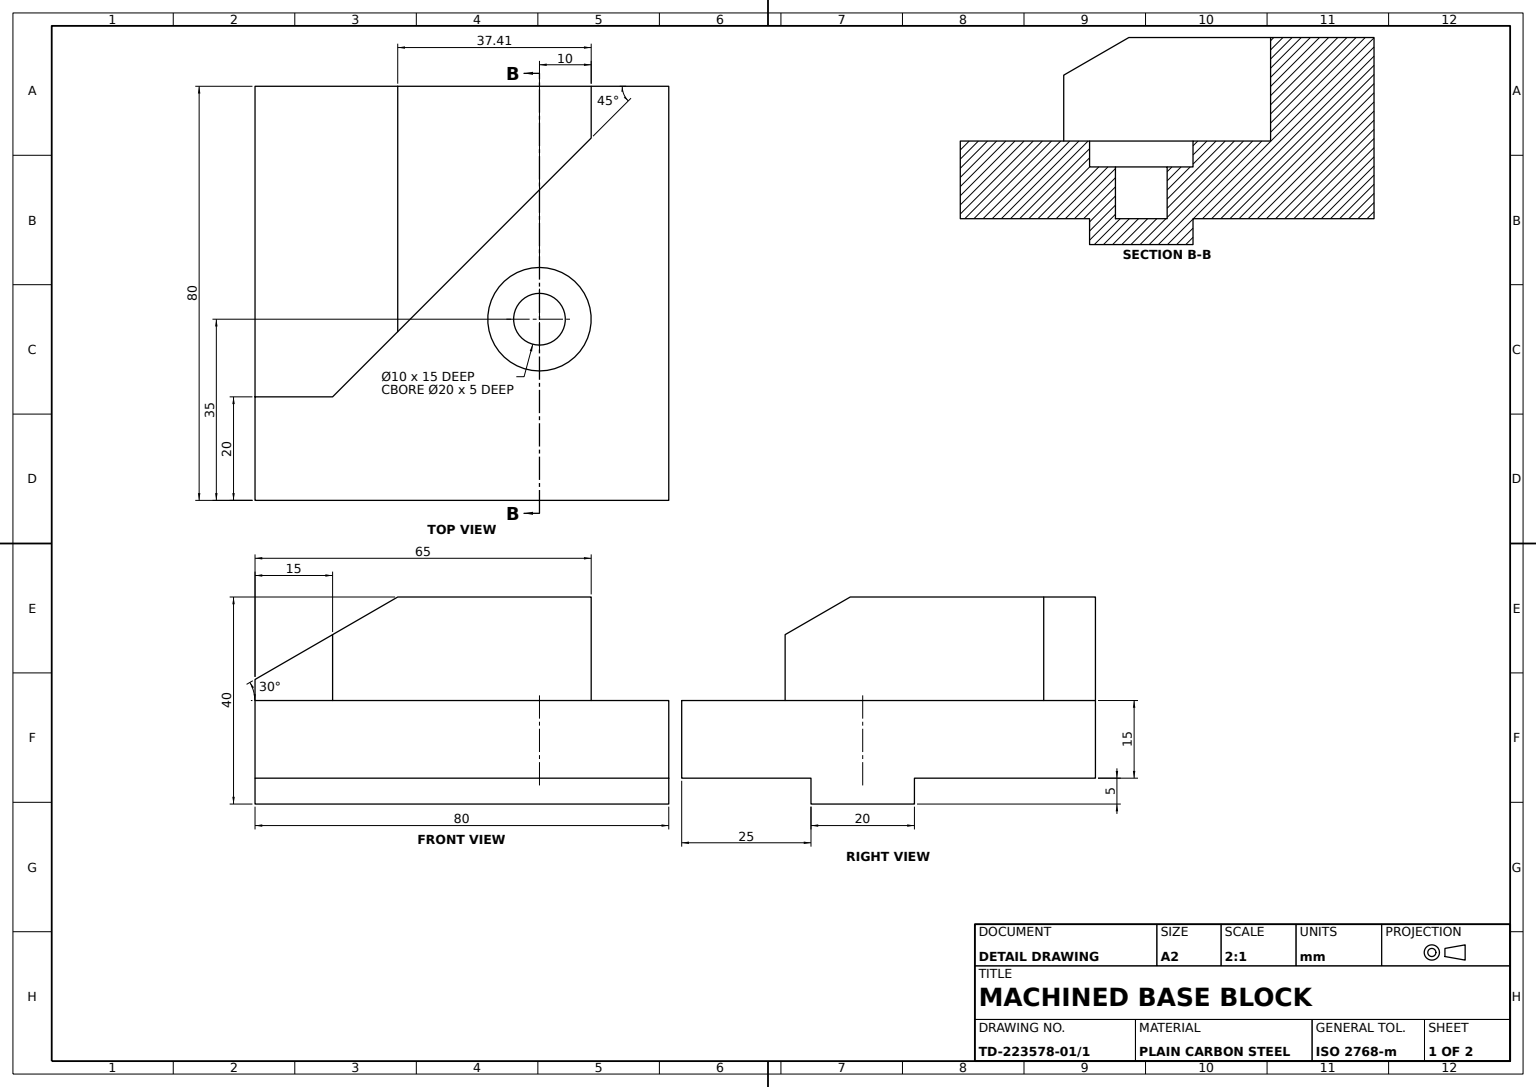
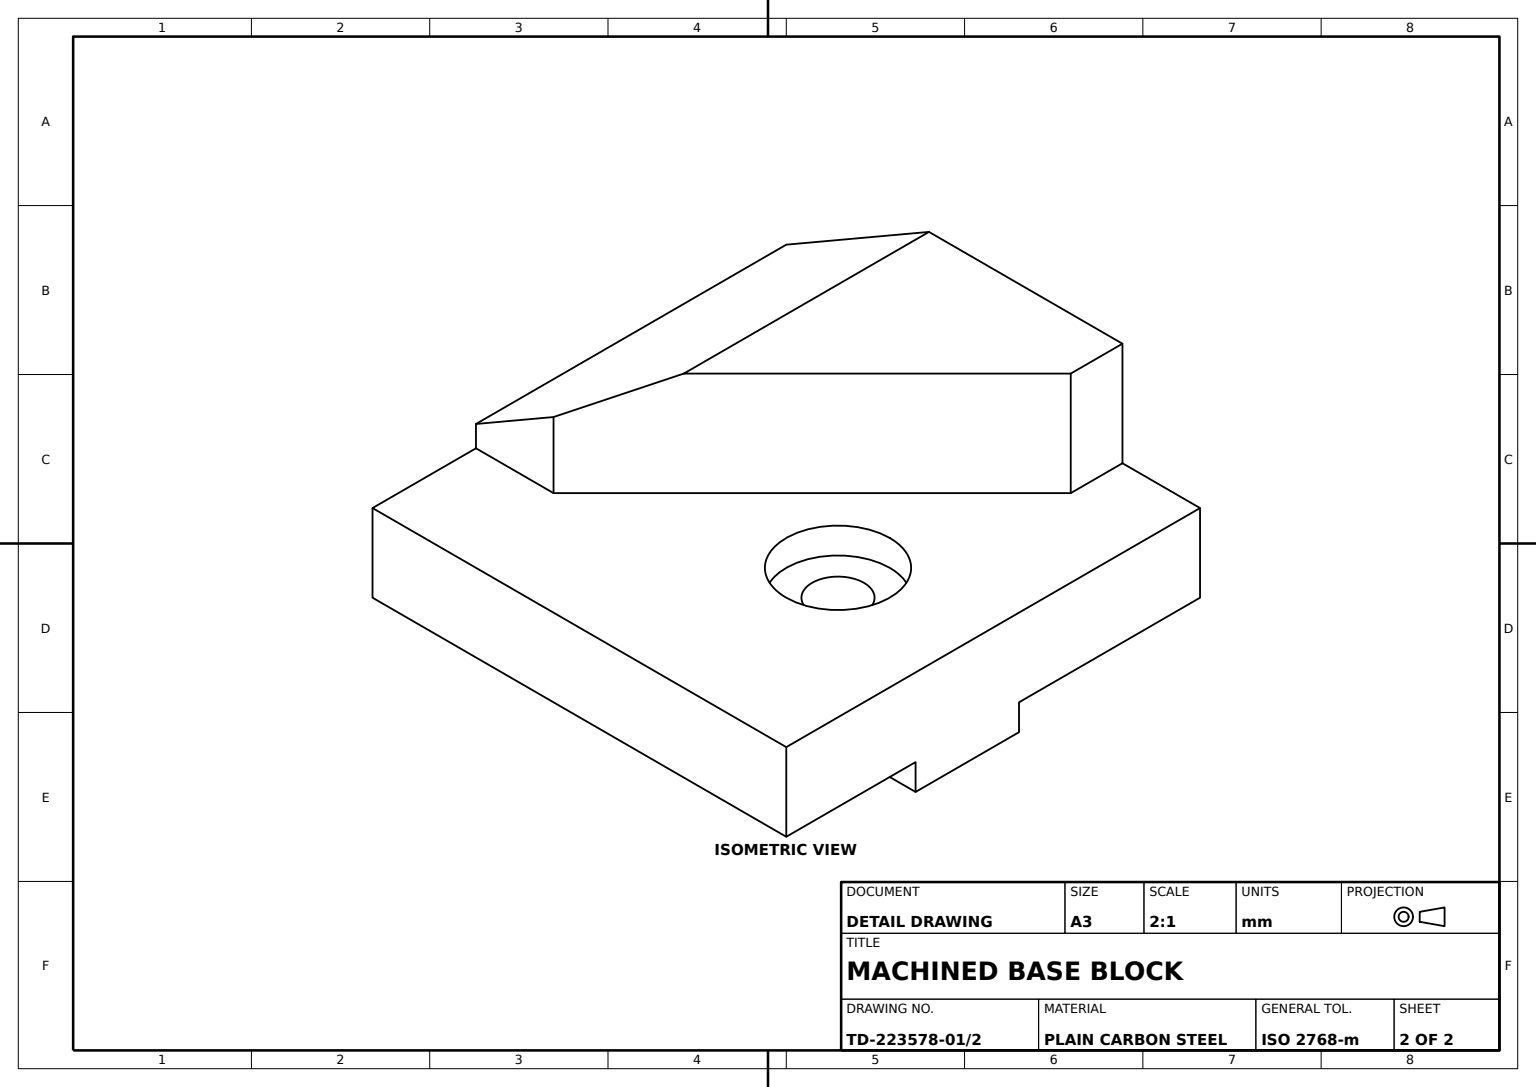
from build123d import *

# Parameters (mm, degrees)
BASE_PLATE_SKETCH_W          = 80
BASE_PLATE_SKETCH_H          = 80
BASE_PLATE_80X80X20_DEPTH    = 20
BOTTOM_SLOT_SKETCH_W         = 25
BOTTOM_SLOT_SKETCH_H         = 5
BOTTOM_SLOT_SKETCH_W_2       = 35
BOTTOM_SLOT_DEPTH            = 80
RAISED_BLOCK_SKETCH_W        = 80
RAISED_BLOCK_SKETCH_H        = 60
RAISED_BLOCK_DEPTH           = 20
BLOCK_STEP_CUT_1_SKETCH_W    = 15
BLOCK_STEP_CUT_1_SKETCH_H    = 10
BLOCK_STEP_CUT_1_DEPTH       = 20
BLOCK_STEP_CUT_2_DEPTH       = 20
BLOCK_ANGLE_CUT_30DEG_REACH  = 102.233
COUNTERBORE_25_SKETCH_R      = 10
COUNTERBORE_25X5_DEPTH       = 5
HOLE_10_SKETCH_R             = 5
HOLE_10X10_DEPTH             = 10
AUXILIARY_BODY_EXTRUDE_DEPTH = 50
AUXILIARY_BODY_FILLET_R20_R  = 20


with BuildPart() as part:
    # Base Plate Sketch → Base Plate 80x80x20 (new body)
    with BuildSketch(Plane(origin=(0, 0, 0), x_dir=(1, 0, 0), z_dir=(0, 1, 0))):
        with Locations((5.239833721, 5.239833721)):
            Rectangle(BASE_PLATE_SKETCH_W, BASE_PLATE_SKETCH_H)
    extrude(amount=BASE_PLATE_80X80X20_DEPTH)

    # Bottom Slot Sketch → Bottom Slot (cut)
    with BuildSketch(Plane(origin=(45.239833721, 0, 0), x_dir=(0, 0, -1), z_dir=(1, 0, 0))):
        with Locations((-22.260166279, 2.5)):
            Rectangle(BOTTOM_SLOT_SKETCH_W, BOTTOM_SLOT_SKETCH_H)
        with Locations((27.739833721, 2.5)):
            Rectangle(BOTTOM_SLOT_SKETCH_W_2, BOTTOM_SLOT_SKETCH_H)
    extrude(amount=-BOTTOM_SLOT_DEPTH, mode=Mode.SUBTRACT)

    # Raised Block Sketch → Raised Block (add)
    with BuildSketch(Plane(origin=(0, 20, 0), x_dir=(1, 0, 0), z_dir=(0, 1, 0))):
        with Locations((5.239833721, 15.239833721)):
            Rectangle(RAISED_BLOCK_SKETCH_W, RAISED_BLOCK_SKETCH_H)
    extrude(amount=RAISED_BLOCK_DEPTH)

    # Block Step Cut 1 Sketch → Block Step Cut 1 (cut)
    with BuildSketch(Plane(origin=(0, 40, 0), x_dir=(1, 0, 0), z_dir=(0, 1, 0))):
        with Locations((37.739833721, 40.239833721)):
            Rectangle(BLOCK_STEP_CUT_1_SKETCH_W, BLOCK_STEP_CUT_1_SKETCH_H)
    extrude(amount=-BLOCK_STEP_CUT_1_DEPTH, mode=Mode.SUBTRACT)

    # Block Step Cut 2 Sketch → Block Step Cut 2 (cut)
    with BuildSketch(Plane(origin=(0, 40, 0), x_dir=(1, 0, 0), z_dir=(0, 1, 0))):
        Polygon((30.239833721, 35.239833721), (-19.760166279, -14.760166279), (45.239833721, -14.760166279), (45.239833721, 35.239833721), align=None)
    extrude(amount=-BLOCK_STEP_CUT_2_DEPTH, mode=Mode.SUBTRACT)

    # Block Angle Cut 30deg Sketch → Block Angle Cut 30deg (cut, up to next)
    with BuildSketch(Plane(origin=(0, 0, -45.239833721), x_dir=(-1, 0, 0), z_dir=(0, 0, -1)), mode=Mode.PRIVATE) as block_angle_cut_30deg_sk1:
        Polygon((34.760166279, 40), (7.167951709, 40), (34.760166279, 24.06962749), align=None)
    block_angle_cut_30deg_tool1 = extrude(block_angle_cut_30deg_sk1.sketch, amount=-BLOCK_ANGLE_CUT_30DEG_REACH, mode=Mode.PRIVATE) & part.part
    add(block_angle_cut_30deg_tool1.solids().sort_by_distance((-25.562761, 34.689876, -45.239834))[0], mode=Mode.SUBTRACT)

    # Counterbore Ø25 Sketch → Counterbore Ø25x5 (cut)
    with BuildSketch(Plane(origin=(0, 20, 0), x_dir=(1, 0, 0), z_dir=(0, 1, 0))):
        with Locations(Location((20.239833721, 0.239833721, 0), (0, 0, 270))):
            Circle(COUNTERBORE_25_SKETCH_R)
    extrude(amount=-COUNTERBORE_25X5_DEPTH, mode=Mode.SUBTRACT)

    # Hole Ø10 Sketch → Hole Ø10x10 (cut)
    with BuildSketch(Plane(origin=(0, 15, 0), x_dir=(1, 0, 0), z_dir=(0, 1, 0))):
        with Locations(Location((20.239833721, 0.239833721, 0), (0, 0, 270))):
            Circle(HOLE_10_SKETCH_R)
    extrude(amount=-HOLE_10X10_DEPTH, mode=Mode.SUBTRACT)


with BuildPart() as body_2:
    # Auxiliary Body Profile Sketch → Auxiliary Body Extrude (new, symmetric)
    with BuildSketch(Plane.XY):
        Polygon((417.503137043, -16.766117227), (417.503137043, -472.594475264), (451.565036325, -472.594475264), (451.565036325, -269.453576574), (494.657405519, -220.272068254), (589.816274586, -472.594475264), (625.881815002, -472.594475264), (519.87061451, -191.49612321), (672.967381657, -16.766117227), (635.900020673, -16.766117227), (451.565036325, -227.148436321), (451.565036325, -16.766117227), align=None)
    extrude(amount=AUXILIARY_BODY_EXTRUDE_DEPTH, both=True)

    # Auxiliary Body Fillet R20
    auxiliary_body_fillet_r20_edges = [body_2.edges().sort_by_distance(p)[0] for p in [
        (451.565036325, -227.148436321, 0),
        (519.87061451, -191.49612321, 0),
        (451.565036325, -269.453576574, 0),
    ]]
    fillet(auxiliary_body_fillet_r20_edges, radius=AUXILIARY_BODY_FILLET_R20_R)


solid = part.part
